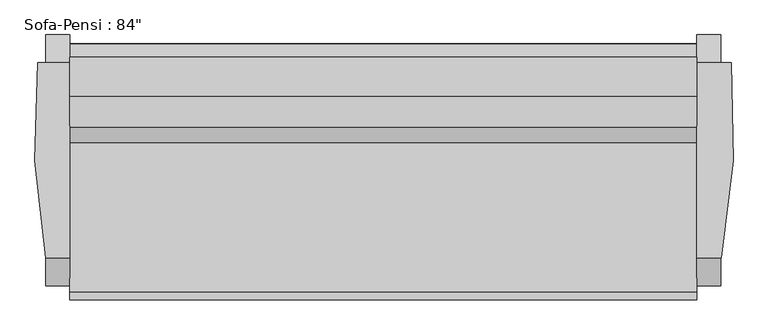
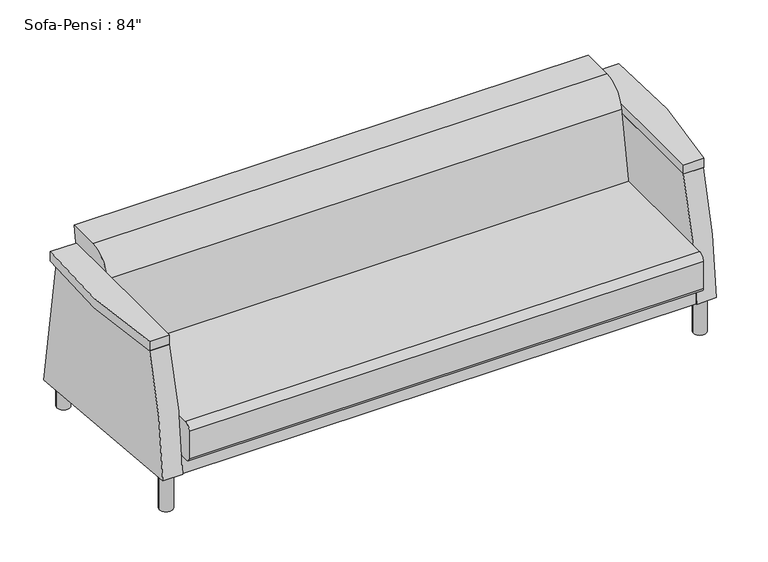
"""IFC4 building model written with IfcOpenShell, lengths in millimetres: furniture geometry."""

from ifc_helpers import new_model, si_unit, point, frame, frame_2d, origin, origin_with_axes, place, context, project, spatial, polyline, circle_curve, trimmed, segment, composite_curve, outline, extrude, source, transform, mapped, element, save


def furniture_aff9b2fb(model_context):
    return source(origin(), model_context, "Body", "SweptSolid", [
        extrude(outline(composite_curve([segment(trimmed(circle_curve(frame_2d((-750.09375, -53.0901639)), 25.4), [point((-775.49375, -53.0901639))], [point((-724.69375, -53.0901639))], False, "CARTESIAN"), True, "CONTINUOUS"), segment(trimmed(circle_curve(frame_2d((-750.09375, -53.0901639)), 25.4), [point((-724.69375, -53.0901639))], [point((-775.49375, -53.0901639))], False, "CARTESIAN"), True, "CONTINUOUS")], self_intersect=False)), origin_with_axes(), (0.0, 0.0, 1.0), 148.43125),
        extrude(outline(composite_curve([segment(trimmed(circle_curve(frame_2d((-750.09375, 632.7098361)), 25.4), [point((-775.49375, 632.7098361))], [point((-724.69375, 632.7098361))], False, "CARTESIAN"), True, "CONTINUOUS"), segment(trimmed(circle_curve(frame_2d((-750.09375, 632.7098361)), 25.4), [point((-724.69375, 632.7098361))], [point((-775.49375, 632.7098361))], False, "CARTESIAN"), True, "CONTINUOUS")], self_intersect=False)), origin_with_axes(), (0.0, 0.0, 1.0), 148.43125),
        extrude(outline(composite_curve([segment(trimmed(circle_curve(frame_2d((1307.30625, 632.7098361)), 25.4), [point((1281.90625, 632.7098361))], [point((1332.70625, 632.7098361))], False, "CARTESIAN"), True, "CONTINUOUS"), segment(trimmed(circle_curve(frame_2d((1307.30625, 632.7098361)), 25.4), [point((1332.70625, 632.7098361))], [point((1281.90625, 632.7098361))], False, "CARTESIAN"), True, "CONTINUOUS")], self_intersect=False)), origin_with_axes(), (0.0, 0.0, 1.0), 148.43125),
        extrude(outline(composite_curve([segment(trimmed(circle_curve(frame_2d((1307.30625, -53.0901639)), 25.4), [point((1281.90625, -53.0901639))], [point((1332.70625, -53.0901639))], False, "CARTESIAN"), True, "CONTINUOUS"), segment(trimmed(circle_curve(frame_2d((1307.30625, -53.0901639)), 25.4), [point((1332.70625, -53.0901639))], [point((1281.90625, -53.0901639))], False, "CARTESIAN"), True, "CONTINUOUS")], self_intersect=False)), origin_with_axes(), (0.0, 0.0, 1.0), 148.43125),
        extrude(outline(polyline([(1269.20625, 668.3047863), (1269.20625, -93.6952137), (-711.99375, -93.6952137), (-711.99375, 668.3047863), (1269.20625, 668.3047863)])), frame((0.0, 0.0, 148.0509954), z_axis=(0.0, 0.0, 1.0), x_axis=(1.0, 0.0, 0.0)), (0.0, 0.0, 1.0), 76.2),
        extrude(outline(composite_curve([segment(polyline([(-9.3943348, 626.0203985), (608.6917937, 626.0203985), (696.2098361, 79.844579), (-97.7900405, 149.3105671)]), True, "CONTINUOUS"), segment(trimmed(circle_curve(frame_2d((1499.9783711, 99.5888442)), 1598.5418814), [point((-97.7900405, 149.3105671))], [point((-9.3943348, 626.0203985))], False, "CARTESIAN"), True, "CONTINUOUS")], self_intersect=False)), frame((-788.19375, 0.0, 0.0), z_axis=(1.0, 0.0, 0.0), x_axis=(0.0, 1.0, 0.0)), (0.0, 0.0, 1.0), 76.2),
        extrude(outline(composite_curve([segment(polyline([(696.2098361, 79.844579), (-97.7900405, 149.3105671)]), True, "CONTINUOUS"), segment(trimmed(circle_curve(frame_2d((1499.9783711, 99.5888442)), 1598.5418814), [point((-97.7900405, 149.3105671))], [point((-9.3943348, 626.0203985))], False, "CARTESIAN"), True, "CONTINUOUS"), segment(polyline([(-9.3943348, 626.0203985), (608.6917937, 626.0203985), (696.2098361, 79.844579)]), True, "CONTINUOUS")], self_intersect=False)), frame((1269.20625, 0.0, 0.0), z_axis=(1.0, 0.0, 0.0), x_axis=(0.0, 1.0, 0.0)), (0.0, 0.0, 1.0), 76.2),
        extrude(outline(composite_curve([segment(trimmed(circle_curve(frame_2d((-116.5901639, 351.2509954)), 25.4), [point((-141.9901639, 351.2509954))], [point((-116.5901639, 376.6509954))], False, "CARTESIAN"), True, "CONTINUOUS"), segment(polyline([(-116.5901639, 376.6509954), (355.3895541, 376.6509954), (402.1988177, 642.1195211)]), True, "CONTINUOUS"), segment(trimmed(circle_curve(frame_2d((502.2552854, 624.4768662)), 101.6), [point((402.1988177, 642.1195211))], [point((502.2552854, 726.0768662))], False, "CARTESIAN"), True, "CONTINUOUS"), segment(polyline([(502.2552854, 726.0768662), (626.3344485, 726.0768662), (609.5377828, 620.1719187), (667.6541767, 224.2509954), (-126.1151639, 224.2509954)]), True, "CONTINUOUS"), segment(trimmed(circle_curve(frame_2d((-126.1151639, 240.1259954)), 15.875), [point((-126.1151639, 224.2509954))], [point((-141.9901639, 240.1259954))], False, "CARTESIAN"), True, "CONTINUOUS"), segment(polyline([(-141.9901639, 240.1259954), (-141.9901639, 351.2509954)]), True, "CONTINUOUS")], self_intersect=False)), frame((-711.99375, 0.0, 0.0), z_axis=(1.0, 0.0, 0.0), x_axis=(0.0, 1.0, 0.0)), (0.0, 0.0, 1.0), 1981.2),
        extrude(outline(composite_curve([segment(polyline([(-711.99375, -9.3943348), (-788.19375, -9.3943348)]), True, "CONTINUOUS"), segment(trimmed(circle_curve(frame_2d((1379.5527561, 389.2532985)), 2204.0972869), [point((-788.19375, -9.3943348))], [point((-813.59375, 608.6917935))], False, "CARTESIAN"), True, "CONTINUOUS"), segment(polyline([(-813.59375, 608.6917935), (-711.99375, 608.6917935), (-711.99375, -9.3943348)]), True, "CONTINUOUS")], self_intersect=False)), frame((0.0, 0.0, 626.0203985), z_axis=(0.0, 0.0, 1.0), x_axis=(1.0, 0.0, 0.0)), (0.0, 0.0, 1.0), 38.1),
        extrude(outline(composite_curve([segment(polyline([(1269.20625, -9.3943348), (1269.20625, 608.9395268), (1377.8864453, 608.9395268)]), True, "CONTINUOUS"), segment(trimmed(circle_curve(frame_2d((-821.3771494, 407.0073811)), 2208.514648), [point((1377.8864453, 608.9395268))], [point((1347.5273117, -9.3943348))], False, "CARTESIAN"), True, "CONTINUOUS"), segment(polyline([(1347.5273117, -9.3943348), (1269.20625, -9.3943348)]), True, "CONTINUOUS")], self_intersect=False)), frame((0.0, 0.0, 626.0203985), z_axis=(0.0, 0.0, 1.0), x_axis=(1.0, 0.0, 0.0)), (0.0, 0.0, 1.0), 38.1),
    ])


if __name__ == "__main__":
    model = new_model("IFC4")
    model_context = context("Model", 3, world=origin())
    ifc_project = project(units=[si_unit("LENGTHUNIT", "METRE", prefix="MILLI")], contexts=[model_context])
    site = spatial("IfcSite", under=ifc_project)
    building = spatial("IfcBuilding", under=site)
    placement = place(None, origin())
    furniture_shape = furniture_aff9b2fb(model_context)
    element("IfcFurniture", 1, ObjectType="Sofa-Pensi : 84\"", at=placement, inside=building, context=model_context, shape_type="MappedRepresentation", body=[
        mapped(furniture_shape, transform((0.0, 0.0, 0.0), x_axis=(1.0, 0.0, 0.0), y_axis=(0.0, 1.0, 0.0), z_axis=(0.0, 0.0, 1.0))),
    ])
    save(model, "model.ifc")

# Revit data of these elements
# Type "Sofa-Pensi : 84\""
#   Assembly Code = "E2020200"
#   Length = 7' - 0"
#   Frame Material = Cherry
#   Seat Material = Linen, Beige
#   Feet Material = Steel, Chrome Plated
# Element 1 (IfcFurniture, "Sofa-Pensi : 84\"")
#   Materials on its faces: "Cherry", "Linen, Beige", "Steel, Chrome Plated"
# Materials
#   "Cherry": class "Wood", colour RGB 226 177 128, transparency 0, Description = "Prunus Serotina", Cost = 0
#   "Linen, Beige": class "Textile", colour RGB 249 239 230, transparency 0, Description = "Linen, beige", Cost = 0
#   "Steel, Chrome Plated": class "Metal", colour RGB 17 17 17, transparency 0, Description = "Chromiuim plated steel", Cost = 0
